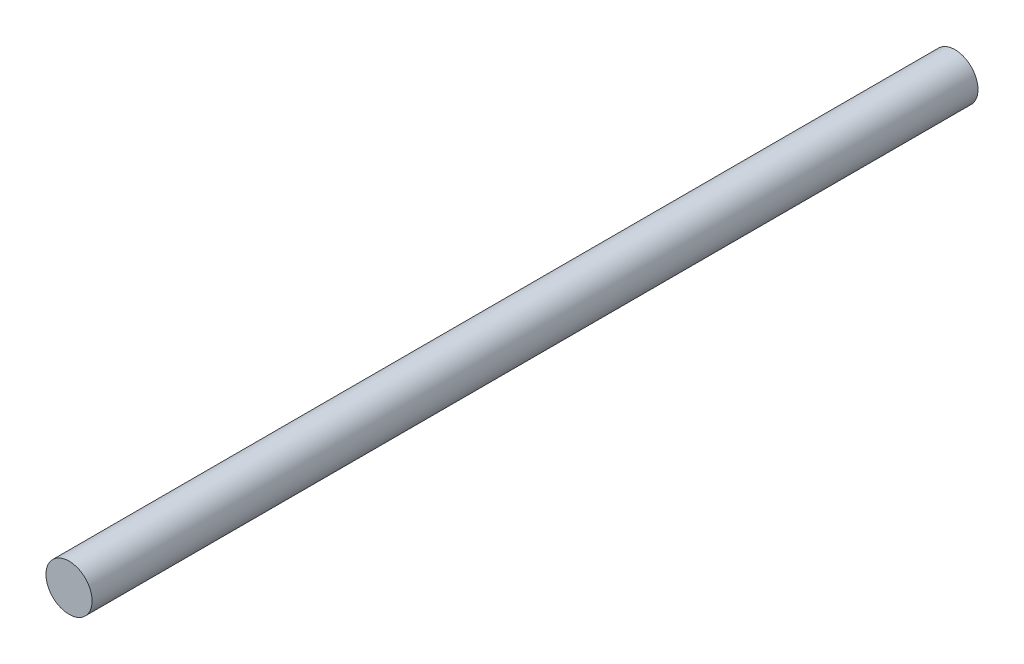
ISO-10303-21;
HEADER;
FILE_DESCRIPTION(('STEP AP214'),'2;1');
FILE_NAME('part.step','',(''),(''),'','','');
FILE_SCHEMA(('AUTOMOTIVE_DESIGN { 1 0 10303 214 1 1 1 1 }'));
ENDSEC;
DATA;
#1=APPLICATION_CONTEXT('core data for automotive mechanical design processes');
#2=APPLICATION_PROTOCOL_DEFINITION('international standard','automotive_design',2000,#1);
#3=PRODUCT_CONTEXT('',#1,'mechanical');
#4=PRODUCT('Part','Part','',(#3));
#5=PRODUCT_RELATED_PRODUCT_CATEGORY('part','',(#4));
#6=PRODUCT_DEFINITION_FORMATION('','',#4);
#7=PRODUCT_DEFINITION_CONTEXT('part definition',#1,'design');
#8=PRODUCT_DEFINITION('design','',#6,#7);
#9=PRODUCT_DEFINITION_SHAPE('','',#8);
#10=(LENGTH_UNIT() NAMED_UNIT(*) SI_UNIT(.MILLI.,.METRE.));
#11=(NAMED_UNIT(*) PLANE_ANGLE_UNIT() SI_UNIT($,.RADIAN.));
#12=(NAMED_UNIT(*) SI_UNIT($,.STERADIAN.) SOLID_ANGLE_UNIT());
#13=UNCERTAINTY_MEASURE_WITH_UNIT(LENGTH_MEASURE(1.E-05),#10,'distance_accuracy_value','');
#14=(GEOMETRIC_REPRESENTATION_CONTEXT(3) GLOBAL_UNCERTAINTY_ASSIGNED_CONTEXT((#13)) GLOBAL_UNIT_ASSIGNED_CONTEXT((#10,
#11,#12)) REPRESENTATION_CONTEXT('',''));
#15=CARTESIAN_POINT('',(0.,0.,0.));
#16=DIRECTION('',(0.,0.,1.));
#17=DIRECTION('',(1.,0.,0.));
#18=AXIS2_PLACEMENT_3D('',#15,#16,#17);
#19=CARTESIAN_POINT('',(0.,0.,48.));
#20=DIRECTION('',(0.,0.,-1.));
#21=DIRECTION('',(-1.,0.,0.));
#22=AXIS2_PLACEMENT_3D('',#19,#20,#21);
#23=CYLINDRICAL_SURFACE('',#22,2.5);
#24=CARTESIAN_POINT('',(0.,0.,48.));
#25=DIRECTION('',(0.,0.,1.));
#26=DIRECTION('',(1.,0.,0.));
#27=AXIS2_PLACEMENT_3D('',#24,#25,#26);
#28=CIRCLE('',#27,2.5);
#29=CARTESIAN_POINT('',(2.5,0.,48.));
#30=VERTEX_POINT('',#29);
#31=EDGE_CURVE('E10',#30,#30,#28,.T.);
#32=ORIENTED_EDGE('',*,*,#31,.F.);
#33=EDGE_LOOP('',(#32));
#34=FACE_BOUND('',#33,.T.);
#35=CARTESIAN_POINT('',(0.,0.,-48.));
#36=DIRECTION('',(0.,0.,1.));
#37=DIRECTION('',(1.,0.,0.));
#38=AXIS2_PLACEMENT_3D('',#35,#36,#37);
#39=CIRCLE('',#38,2.5);
#40=CARTESIAN_POINT('',(2.5,0.,-48.));
#41=VERTEX_POINT('',#40);
#42=EDGE_CURVE('E37',#41,#41,#39,.T.);
#43=ORIENTED_EDGE('',*,*,#42,.T.);
#44=EDGE_LOOP('',(#43));
#45=FACE_BOUND('',#44,.T.);
#46=ADVANCED_FACE('F40',(#34,#45),#23,.T.);
#47=CARTESIAN_POINT('',(0.,0.,48.));
#48=DIRECTION('',(0.,0.,1.));
#49=DIRECTION('',(1.,0.,0.));
#50=AXIS2_PLACEMENT_3D('',#47,#48,#49);
#51=PLANE('',#50);
#52=ORIENTED_EDGE('',*,*,#31,.T.);
#53=EDGE_LOOP('',(#52));
#54=FACE_BOUND('',#53,.T.);
#55=ADVANCED_FACE('F55',(#54),#51,.T.);
#56=CARTESIAN_POINT('',(0.,0.,-48.));
#57=DIRECTION('',(0.,0.,1.));
#58=DIRECTION('',(1.,0.,0.));
#59=AXIS2_PLACEMENT_3D('',#56,#57,#58);
#60=PLANE('',#59);
#61=ORIENTED_EDGE('',*,*,#42,.F.);
#62=EDGE_LOOP('',(#61));
#63=FACE_BOUND('',#62,.T.);
#64=ADVANCED_FACE('F49',(#63),#60,.F.);
#65=CLOSED_SHELL('',(#46,#55,#64));
#66=MANIFOLD_SOLID_BREP('B2',#65);
#67=ADVANCED_BREP_SHAPE_REPRESENTATION('',(#18,#66),#14);
#68=SHAPE_DEFINITION_REPRESENTATION(#9,#67);
ENDSEC;
END-ISO-10303-21;
